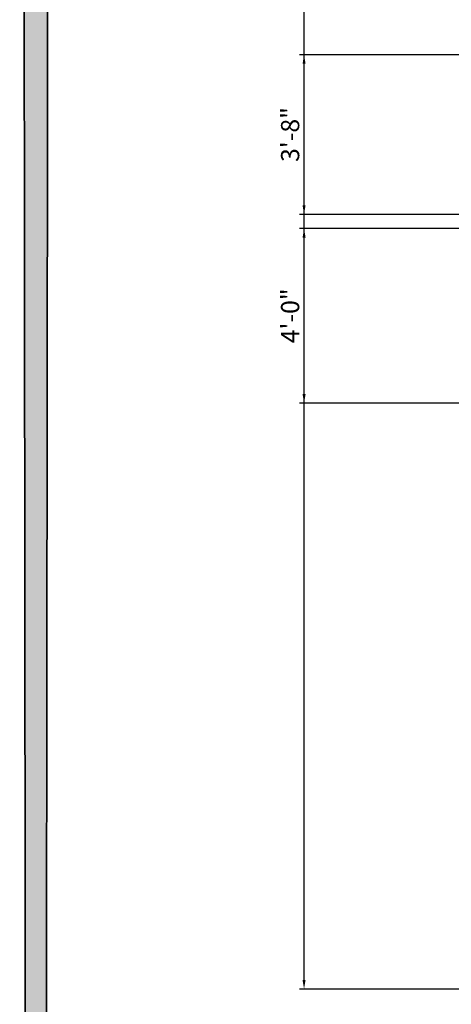
# Model space of a CAD drawing. Units: inches. Extents: x 1804 to 3296, y 909 to 2477.
# Tile 2 of 31: x 1804 to 1922, y 1059 to 1329. Entities that reach past the tile are written whole.
import ezdxf

# ---------------------------------------------------------------- set-up
doc = ezdxf.new("R2010")
doc.units = ezdxf.units.IN
doc.layers.add('A-ANNO-DIMS', color=2, linetype='Continuous', lineweight=18)
doc.layers.add('A-ANNO-TTLB', color=156, linetype='Continuous', lineweight=35)
doc.styles.get("Standard").update_dxf_attribs({"font": 'arial.ttf'})
doc.dimstyles.new('ISO-25', dxfattribs={"dimtxt": 5, "dimasz": 2.5, "dimexe": 1.25, "dimexo": 0.625, "dimtad": 1, "dimdec": 0, "dimlunit": 4, "dimtxsty": 'Standard', "dimcen": 2.5, "dimadec": 0, "dimazin": 0, "dimtfac": 1, "dimtdec": 0, "dimtmove": 0, "dimatfit": 3, "dimfxl": 1, "dimarcsym": 0})

# ---------------------------------------------------------------- blocks, each defined once
blk = doc.blocks.new('*D52')
at = {"layer": 'A-ANNO-DIMS', "color": 0, "lineweight": -2, "transparency": 16777216}
for p, q in [((1924.96, 1830.04), (1880.63, 1830.04)), ((1881.88, 1065.27), (1881.88, 1827.54)), ((1924.96, 1062.77), (1880.63, 1062.77))]:
    blk.add_line(p, q, dxfattribs=at)
at = {"layer": 'A-ANNO-DIMS', "color": 0, "lineweight": 100, "transparency": 16777216}
for points in [[(1881.47, 1827.54), (1882.3, 1827.54), (1881.88, 1830.04)], [(1881.47, 1065.27), (1882.3, 1065.27), (1881.88, 1062.77)]]:
    blk.add_solid(points, dxfattribs=at)
at = {"layer": 'Defpoints', "color": 0, "lineweight": 100, "transparency": 16777216}
for p in [(1881.88, 1830.04), (1925.58, 1830.04), (1925.58, 1062.77)]:
    blk.add_point(p, dxfattribs=at)
at = {"layer": 'A-ANNO-DIMS', "color": 0, "transparency": 16777216, "insert": (1878.67, 1446.4), "char_height": 5, "attachment_point": 5, "rotation": 90}
blk.add_mtext('63\'-11 1/2"', dxfattribs=at)
blk = doc.blocks.new('*D63')
at = {"layer": 'A-ANNO-DIMS', "color": 0, "lineweight": -2, "transparency": 16777216}
for p, q in [((2157.95, 1319.33), (1880.63, 1319.33)), ((1881.88, 1277.99), (1881.88, 1316.83)), ((2157.95, 1275.49), (1880.63, 1275.49))]:
    blk.add_line(p, q, dxfattribs=at)
at = {"layer": 'A-ANNO-DIMS', "color": 0, "lineweight": 100, "transparency": 16777216}
for points in [[(1881.47, 1316.83), (1882.3, 1316.83), (1881.88, 1319.33)], [(1881.47, 1277.99), (1882.3, 1277.99), (1881.88, 1275.49)]]:
    blk.add_solid(points, dxfattribs=at)
at = {"layer": 'Defpoints', "color": 0, "lineweight": 100, "transparency": 16777216}
for p in [(1881.88, 1319.33), (2158.58, 1319.33), (2158.58, 1275.49)]:
    blk.add_point(p, dxfattribs=at)
at = {"layer": 'A-ANNO-DIMS', "color": 0, "transparency": 16777216, "insert": (1878.7, 1297.41), "char_height": 5, "attachment_point": 5, "rotation": 90}
blk.add_mtext('3\'-8"', dxfattribs=at)
blk = doc.blocks.new('*D70')
at = {"layer": 'A-ANNO-DIMS', "color": 0, "lineweight": -2, "transparency": 16777216}
for p, q in [((2208.56, 1271.63), (1880.63, 1271.63)), ((1881.88, 1226.13), (1881.88, 1269.13)), ((2208.56, 1223.63), (1880.63, 1223.63))]:
    blk.add_line(p, q, dxfattribs=at)
at = {"layer": 'A-ANNO-DIMS', "color": 0, "lineweight": 100, "transparency": 16777216}
for points in [[(1881.47, 1269.13), (1882.3, 1269.13), (1881.88, 1271.63)], [(1881.47, 1226.13), (1882.3, 1226.13), (1881.88, 1223.63)]]:
    blk.add_solid(points, dxfattribs=at)
at = {"layer": 'Defpoints', "color": 0, "lineweight": 100, "transparency": 16777216}
for p in [(1881.88, 1271.63), (2209.19, 1271.63), (2209.19, 1223.63)]:
    blk.add_point(p, dxfattribs=at)
at = {"layer": 'A-ANNO-DIMS', "color": 0, "transparency": 16777216, "insert": (1878.7, 1247.63), "char_height": 5, "attachment_point": 5, "rotation": 90}
blk.add_mtext('4\'-0"', dxfattribs=at)

msp = doc.modelspace()

# ---------------------------------------------------------------- hatches: boundary and pattern name
at = {"layer": 'A-ANNO-TTLB'}
h = msp.add_hatch(color=256, dxfattribs=at)
h.dxf.hatch_style = 1
h.paths.add_polyline_path([(3294.53, 2476.54), (1803.79, 2476.54), (1805.43, 909.47), (3296.17, 909.47)])
h.paths.add_polyline_path([(1811, 914.33), (1812.79, 2467.54), (3285.53, 2467.54), (3283.74, 914.33)], flags=16)
h.paths.add_polyline_path([(1925.58, 1062.77), (1925.58, 1138.07), (1925.58, 1539.88), (1925.58, 1793.38), (1925.58, 1830.04), (2325.54, 1830.04), (2325.54, 1793.38), (2325.54, 1586.42), (2325.54, 1138.07), (2325.54, 1062.77)], flags=0)
h.paths.add_polyline_path([(1997.22, 1029.4), (2008.85, 1037.96), (2008.85, 1020.84)], flags=0)
h.paths.add_polyline_path([(1934.58, 1138.07), (1934.58, 1147.07), (2078.77, 1147.07), (2078.77, 1138.07), (2060.94, 1138.07)], flags=0)
h.paths.add_polyline_path([(1944.35, 1138.07), (1944.35, 1147.07), (2056.05, 1147.07), (2056.05, 1138.07)], flags=0)
h.paths.add_polyline_path([(2222.24, 1037.96), (2233.87, 1029.4), (2222.24, 1020.84)], flags=0)
h.paths.add_polyline_path([(2061.94, 1139.07), (2061.94, 1146.07), (2077.77, 1146.07), (2077.77, 1139.07)], flags=0)
h.paths.add_polyline_path([(2149.58, 1138.07), (2149.58, 1269.44), (2158.58, 1269.44), (2158.58, 1326.69), (2149.58, 1326.69), (2149.58, 1340.94), (2139.6, 1340.94), (2139.6, 1434.25), (2149.58, 1434.25), (2149.58, 1447.36), (2158.58, 1447.36), (2158.58, 1423.87), (2158.58, 1408.06), (2198.46, 1408.06), (2198.46, 1412.56), (2282.65, 1412.56), (2282.65, 1465.94), (2316.54, 1465.94), (2316.54, 1590.92), (2192.86, 1590.92), (2192.86, 1595.3), (2291.17, 1595.3), (2291.17, 1590.92), (2316.54, 1590.92), (2316.54, 1784.38), (2300.24, 1784.38), (2300.24, 1757.47), (2268, 1757.47), (2268, 1681.04), (2180.87, 1681.04), (2180.87, 1757.47), (2148.63, 1757.47), (2148.63, 1784.38), (2119.08, 1784.38), (2119.08, 1585.58), (2114.58, 1585.58), (2114.58, 1784.38), (2064.11, 1784.38), (2046.28, 1784.38), (2046.28, 1760.38), (1958.58, 1760.38), (1958.58, 1664.38), (1934.58, 1664.38), (1934.58, 1784.38), (1934.58, 1793.38), (2046.28, 1793.38), (2064.11, 1793.38), (2119.08, 1793.38), (2230.78, 1793.38), (2230.78, 1784.38), (2268, 1784.38), (2300.24, 1784.38), (2316.54, 1784.38), (2316.54, 1590.92), (2316.54, 1373.73), (2316.54, 1138.07)], flags=0)
h.paths.add_polyline_path([(2209.19, 1166.63), (2209.19, 1175.63), (2158.58, 1175.63), (2209.19, 1223.63), (2209.19, 1231.63), (2183.88, 1231.63), (2183.88, 1301.66), (2242.59, 1301.66), (2242.59, 1326.69), (2316.54, 1326.69), (2272.59, 1271.63), (2272.59, 1223.63), (2316.54, 1175.63), (2272.59, 1175.63), (2272.59, 1166.63)], flags=0)
h.paths.add_polyline_path([(1947.77, 1345.22), (1947.77, 1457.48), (1991.2, 1457.48), (1991.2, 1451.7), (1991.2, 1352.18), (1991.2, 1345.22)], flags=0)
h.paths.add_polyline_path([(2209.19, 1271.63), (2262.59, 1271.63), (2262.59, 1311.85), (2272.59, 1301.66), (2272.59, 1271.63), (2269.92, 1269.63), (2270.59, 1269.63), (2270.59, 1225.63), (2211.19, 1225.63), (2211.19, 1269.63), (2211.86, 1269.63)], flags=0)
h.paths.add_polyline_path([(2000.34, 1378.21), (2000.34, 1429.71), (2025.22, 1429.71), (2025.22, 1378.21)], flags=0)
h.paths.add_polyline_path([(2001.34, 1379.21), (2001.34, 1428.71), (2024.22, 1428.71), (2024.22, 1379.21)], flags=0)
h.paths.add_polyline_path([(2012.34, 1390.21), (2012.34, 1417.71), (2013.22, 1417.71), (2013.22, 1390.21)], flags=0)
h.paths.add_polyline_path([(2237.56, 1331.19), (2237.56, 1340.18), (2238.62, 1340.18), (2238.62, 1386.84), (2241.04, 1386.84), (2242.06, 1386.84), (2242.06, 1408.06), (2316.54, 1331.19)], flags=0)
h.paths.add_polyline_path([(1953.73, 1464.35), (1953.73, 1498.59), (1981.74, 1498.59), (1981.74, 1464.35)], flags=0)
h.paths.add_polyline_path([(1987.63, 1462.08), (1987.63, 1500.95), (2104.07, 1500.95), (2104.07, 1462.08), (2099.27, 1462.08), (1993.6, 1462.08)], flags=0)
h.paths.add_polyline_path([(1956.06, 1481.47, -1), (1979.41, 1481.47, -1)], flags=0)
edge = h.paths.add_edge_path(flags=0)
edge.add_ellipse((2299.53, 1438.37), major_axis=(0.31, 21.36), ratio=0.670333, start_angle=0, end_angle=360)
h.paths.add_polyline_path([(2297.39, 1438.37, -1), (2301.67, 1438.37, -1)], flags=0)
h.paths.add_polyline_path([(2591.54, 1163.23), (2591.54, 1179.38), (2591.54, 1379.68), (2591.54, 1395.84), (2734.5, 1395.84), (2734.5, 1379.68), (2734.5, 1179.38), (2734.5, 1163.23)], flags=0)
h.paths.add_polyline_path([(2592.54, 1164.23), (2592.54, 1166.23), (2733.5, 1166.23), (2733.5, 1164.23)], flags=0)
h.paths.add_polyline_path([(2592.54, 1180.38), (2592.54, 1378.68), (2733.5, 1378.68), (2733.5, 1180.38)], flags=0)
h.paths.add_polyline_path([(2593.54, 1181.38), (2593.54, 1377.68), (2732.5, 1377.68), (2732.5, 1181.38)], flags=0)
h.paths.add_polyline_path([(2594.54, 1182.38), (2594.54, 1376.68), (2731.5, 1376.68), (2731.5, 1182.38)], flags=0)
h.paths.add_polyline_path([(1936.95, 1697.46), (1936.95, 1736.46), (1955.41, 1736.46), (1955.41, 1697.46)], flags=0)
h.paths.add_polyline_path([(1938.48, 1718.36), (1938.48, 1734.92), (1953.65, 1734.92), (1953.65, 1718.36)], flags=0)
h.paths.add_polyline_path([(1944.75, 1726.64, -1), (1947.37, 1726.64, -1)], flags=0)
h.paths.add_polyline_path([(2592.54, 1394.84), (2733.5, 1394.84), (2733.5, 1392.84), (2592.54, 1392.84)], flags=0)
h.paths.add_polyline_path([(1976.61, 1762.5), (1976.61, 1781.44), (2012.79, 1781.44), (2012.79, 1762.5)], flags=0)
h.paths.add_polyline_path([(1979.57, 1771.97, -1), (1991.39, 1771.97, -1)], flags=0)
h.paths.add_polyline_path([(1995.36, 1771.97, -1), (2007.18, 1771.97, -1)], flags=0)
h.paths.add_polyline_path([(2251.51, 1744.53), (2268, 1730.05), (2251.51, 1730.05)], flags=0)
h.paths.add_polyline_path([(2047.28, 1785.38), (2047.28, 1792.38), (2063.11, 1792.38), (2063.11, 1785.38)], flags=0)
h.paths.add_polyline_path([(2155.08, 1770.92, -1), (2174.42, 1770.92, -1)], flags=0)
h.paths.add_polyline_path([(2188.59, 1758.27), (2188.59, 1772.81), (2222.3, 1772.81), (2222.3, 1758.27)], flags=0)
h.paths.add_polyline_path([(2223.97, 1758.27), (2223.97, 1772.81), (2257.68, 1772.81), (2257.68, 1758.27)], flags=0)
h.paths.add_polyline_path([(2274.45, 1770.92, -1), (2293.8, 1770.92, -1)], flags=0)
h.paths.add_polyline_path([(2591.54, 1582.09), (2591.54, 1782.39), (2734.5, 1782.39), (2734.5, 1582.09)], flags=0)
h.paths.add_polyline_path([(2592.54, 1583.09), (2592.54, 1781.39), (2733.5, 1781.39), (2733.5, 1583.09)], flags=0)
h.paths.add_polyline_path([(2593.54, 1584.09), (2593.54, 1780.39), (2732.5, 1780.39), (2732.5, 1584.09)], flags=0)
h.paths.add_polyline_path([(2594.54, 1585.09), (2594.54, 1779.39), (2731.5, 1779.39), (2731.5, 1585.09)], flags=0)
h.paths.add_polyline_path([(1922.17, 1978.79), (1922.17, 2295.08), (1922.17, 2296.08), (2115.67, 2296.08), (2115.67, 2384.31), (2115.67, 2385.31), (2322.12, 2385.31), (2323.12, 2385.31), (2323.12, 1979.79), (2323.12, 1978.79), (1923.17, 1978.79)], flags=0)
h.paths.add_polyline_path([(1922.17, 1978.79), (1922.17, 2051.31), (1922.17, 2214.86), (1922.17, 2296.08), (2115.67, 2296.08), (2115.67, 2385.31), (2323.12, 2385.31), (2323.12, 2280.42), (2323.12, 1978.79), (2115.67, 1978.79)], flags=0)
h.paths.add_polyline_path([(1923.17, 1979.79), (1923.17, 2050.31), (2115.67, 2050.31), (2115.67, 2051.31), (1923.17, 2051.31), (1923.17, 2213.86), (1923.17, 2214.86), (1923.17, 2295.08), (1990.02, 2295.08), (1990.02, 2214.86), (1991.02, 2214.86), (1991.02, 2295.08), (2115.67, 2295.08), (2115.67, 1979.79), (2116.67, 1979.79), (2116.67, 2304.18), (2116.67, 2384.31), (2322.12, 2384.31), (2322.12, 2280.42), (2322.12, 1979.79), (2115.67, 1979.79)], flags=0)
h.paths.add_polyline_path([(2972.46, 1192.5), (2972.46, 1196.92), (2995.47, 1196.92), (2995.47, 1255.47), (2995.09, 1255.47), (2987.42, 1249.39), (2980.08, 1255.47), (2978.05, 1255.47), (2978.05, 1257.24), (2995.47, 1257.24), (2995.47, 1261.58), (3015.37, 1261.58), (3015.37, 1333.28), (3015.37, 1414.4), (3032.82, 1414.4), (3032.82, 1333.28), (3032.82, 1261.58), (3052.66, 1261.58), (3052.66, 1255.47), (3079.86, 1255.47), (3078.72, 1254.57), (3081.47, 1252.29), (3078.56, 1249.99), (3075.81, 1252.26), (3072.57, 1249.69), (3070.36, 1251.52), (3067.67, 1249.39), (3060.34, 1255.47), (3052.66, 1255.47), (3052.66, 1196.92), (3054.58, 1196.92), (3074, 1196.92), (3074, 1192.5), (3052.66, 1192.5), (2995.47, 1192.5)], flags=0)
h.paths.add_polyline_path([(2490.75, 1979.27), (2490.75, 1980.27), (2596.87, 1980.27), (2596.87, 2051.8), (2596.87, 2052.8), (2596.87, 2216.35), (2596.87, 2297.57), (2717.32, 2297.57), (2710.57, 2305.62), (2724.07, 2305.62), (2717.32, 2297.57), (2782.37, 2297.57), (2782.37, 2395.8), (3006.82, 2395.8), (3006.82, 1981.27), (3093.73, 1981.27), (3093.73, 1980.27), (3047.51, 1980.27), (3046.37, 1979.37), (3049.11, 1977.1), (3046.2, 1974.79), (3043.46, 1977.07), (3040.21, 1974.49), (3038, 1976.32), (3035.32, 1974.2), (3027.98, 1980.27), (2871.83, 1980.27), (2871.83, 1981.27), (2791.37, 1981.27), (2791.37, 2050.8), (2597.87, 2050.8), (2597.87, 1980.27), (2597.87, 1979.27), (2546.27, 1979.27), (2545.12, 1978.37), (2547.87, 1976.1), (2544.96, 1973.79), (2542.22, 1976.07), (2538.97, 1973.49), (2536.76, 1975.32), (2534.07, 1973.2), (2526.74, 1979.27)], flags=0)
h.paths.add_polyline_path([(2597.87, 2051.8), (2606.87, 2051.8), (2606.87, 2258.39), (2597.87, 2258.39), (2597.87, 2296.57), (2606.87, 2296.57), (2606.87, 2262.39), (2782.37, 2262.39), (2782.37, 2296.57), (2790.37, 2296.57), (2790.37, 2262.39), (2791.37, 2262.39), (2791.37, 2305.67), (2791.37, 2385.8), (2996.82, 2385.8), (2996.82, 2339.85), (3006.82, 2339.85), (3006.82, 2250.12), (2997.82, 2250.12), (2997.82, 1981.27), (2996.82, 1981.27), (2872.83, 1981.27), (2872.83, 1991.8), (2871.83, 1991.8), (2871.83, 2050.8), (2790.37, 2050.8), (2597.87, 2050.8)], flags=0)
h.paths.add_polyline_path([(2179.93, 2153.92), (2179.93, 2353.97), (2259.98, 2353.97), (2259.98, 2153.92)], flags=0)
h.paths.add_polyline_path([(2180.93, 2154.92), (2180.93, 2352.97), (2258.98, 2352.97), (2258.98, 2154.92)], flags=0)
h.paths.add_polyline_path([(2960.87, 1608.49), (2960.87, 1753.62), (3070.9, 1753.62), (3070.9, 1608.49)], flags=0)
h.paths.add_polyline_path([(2961.87, 1609.49), (2961.87, 1752.62), (3069.9, 1752.62), (3069.9, 1609.49)], flags=0)
h.paths.add_polyline_path([(2962.87, 1610.49), (2962.87, 1751.62), (3068.9, 1751.62), (3068.9, 1610.49)], flags=0)
h.paths.add_polyline_path([(2963.87, 1611.49), (2963.87, 1750.62), (3067.9, 1750.62), (3067.9, 1611.49)], flags=0)
h.paths.add_polyline_path([(2782.37, 2051.8), (2782.37, 2216.32), (2791.37, 2216.32), (2791.37, 2051.8), (2872.83, 2051.8), (2872.83, 2068.56), (2884.67, 2068.56), (2884.67, 2085.33), (2896.51, 2085.33), (2896.51, 2102.09), (2908.36, 2102.09), (2908.36, 2118.85), (2920.2, 2118.85), (2920.2, 2135.62), (2932.05, 2135.62), (2932.05, 2145.3), (2925.08, 2145.3), (2925.08, 2203.2), (2996.82, 2203.2), (2996.82, 2145.3), (2953.82, 2145.3), (2872.83, 2051.8), (2790.37, 2051.8)], flags=0)
h.paths.add_polyline_path([(2717.32, 2238.65), (2710.57, 2246.7), (2724.07, 2246.7)], flags=0)
h.paths.add_polyline_path([(2003.09, 1122.79), (2017.16, 1122.79), (2017.16, 1138.74), (2003.09, 1138.74)], flags=8)
h.paths.add_polyline_path([(2174.76, 1792.72), (2188.83, 1792.72), (2188.83, 1808.66), (2174.76, 1808.66)], flags=8)
h.paths.add_polyline_path([(1987.95, 1792.51), (2002.02, 1792.51), (2002.02, 1808.45), (1987.95, 1808.45)], flags=8)
h.paths.add_polyline_path([(2148.79, 1289.26), (2160.46, 1289.26), (2160.46, 1305.2), (2148.79, 1305.2)], flags=8)
h.paths.add_polyline_path([(2115.36, 1133.57), (2127.04, 1133.57), (2127.04, 1149.51), (2115.36, 1149.51)], flags=8)
h.paths.add_polyline_path([(2237.58, 1421.48), (2249.25, 1421.48), (2249.25, 1437.43), (2237.58, 1437.43)], flags=8)
h.paths.add_polyline_path([(2134.99, 1584.32), (2146.66, 1584.32), (2146.66, 1600.26), (2134.99, 1600.26)], flags=8)
h.paths.add_polyline_path([(2101.95, 1557.31), (2113.62, 1557.31), (2113.62, 1573.25), (2101.95, 1573.25)], flags=8)
h.paths.add_polyline_path([(2937.85, 1156.77), (3120.41, 1156.77), (3120.41, 1185.72), (2937.85, 1185.72)], flags=8)
h.paths.add_polyline_path([(2980.71, 1786.71), (3050.06, 1786.71), (3050.06, 1802.66), (2980.71, 1802.66)], flags=8)
h.paths.add_polyline_path([(2869.28, 1661.96), (2938.62, 1661.96), (2938.62, 1690.8), (2869.28, 1690.8)], flags=8)
h.paths.add_polyline_path([(3092.27, 1674.86), (3161.62, 1674.86), (3161.62, 1690.8), (3092.27, 1690.8)], flags=8)
h.paths.add_polyline_path([(2980.71, 1674.86), (3050.06, 1674.86), (3050.06, 1690.8), (2980.71, 1690.8)], flags=8)
h.paths.add_polyline_path([(2649.07, 1678.23), (2674.53, 1678.23), (2674.53, 1714.76), (2649.07, 1714.76)], flags=8)
h.paths.add_polyline_path([(2530.84, 1981.63), (2549.13, 1981.63), (2549.13, 1997.57), (2530.84, 1997.57)], flags=8)
h.paths.add_polyline_path([(3031.29, 1981.77), (3049.58, 1981.77), (3049.58, 1997.71), (3031.29, 1997.71)], flags=8)
h.paths.add_polyline_path([(2715.38, 1911.9), (2851.54, 1911.9), (2851.54, 1940.85), (2715.38, 1940.85)], flags=8)
h.paths.add_polyline_path([(2015.23, 1927.36), (2205.42, 1927.36), (2205.42, 1956.3), (2015.23, 1956.3)], flags=8)
h.paths.add_polyline_path([(2671.84, 2057.84), (2702.75, 2057.84), (2702.75, 2073.79), (2671.84, 2073.79)], flags=8)
h.paths.add_polyline_path([(2678.5, 2316.52), (2765.26, 2316.52), (2765.26, 2332.46), (2678.5, 2332.46)], flags=8)
h.paths.add_polyline_path([(2678.48, 2271.96), (2736.41, 2271.96), (2736.41, 2287.9), (2678.48, 2287.9)], flags=8)
h.paths.add_polyline_path([(2019.2, 972.79), (2243.21, 972.79), (2243.21, 1001.74), (2019.2, 1001.74)], flags=8)
h.paths.add_polyline_path([(2097.06, 1021.56), (2132.16, 1021.56), (2132.16, 1037.51), (2097.06, 1037.51)], flags=8)
h.paths.add_polyline_path([(2182.47, 1360.48), (2207.35, 1360.48), (2207.35, 1376.42), (2182.47, 1376.42)], flags=8)
h.paths.add_polyline_path([(2261.12, 1361.77), (2295.01, 1361.77), (2295.01, 1377.71), (2261.12, 1377.71)], flags=8)
h.paths.add_polyline_path([(2245.75, 1511.51), (2278.44, 1511.51), (2278.44, 1527.46), (2245.75, 1527.46)], flags=8)
h.paths.add_polyline_path([(1991.16, 1296.29), (2060.51, 1296.29), (2060.51, 1312.23), (1991.16, 1312.23)], flags=8)
h.paths.add_polyline_path([(2187, 1651.35), (2246.71, 1651.35), (2246.71, 1667.29), (2187, 1667.29)], flags=8)
h.paths.add_polyline_path([(1976.49, 1684.81), (2068.63, 1684.81), (2068.63, 1700.76), (1976.49, 1700.76)], flags=8)

# ---------------------------------------------------------------- linework, layer by layer
for points in [[(1803.79, 2476.54), (3294.53, 2476.54), (3296.17, 909.47), (1805.43, 909.47)], [(1812.79, 2467.54), (3285.53, 2467.54), (3283.74, 914.33), (1811, 914.33)]]:
    msp.add_lwpolyline(points, close=True, dxfattribs=at)

# ---------------------------------------------------------------- dimensions: what is measured, and where the dimension line sits
at = {"layer": 'A-ANNO-DIMS'}
for base, p1, p2, picture, middle in [((1881.88, 1830.04), (1925.58, 1062.77), (1925.58, 1830.04), '*D52', (1878.67, 1446.4)), ((1881.88, 1319.33), (2158.58, 1275.49), (2158.58, 1319.33), '*D63', (1878.7, 1297.41)), ((1881.88, 1271.63), (2209.19, 1223.63), (2209.19, 1271.63), '*D70', (1878.7, 1247.63))]:
    dim = msp.add_linear_dim(base=base, p1=p1, p2=p2, angle=90, dimstyle='ISO-25', override={"dimdec": 1, "dimlfac": 1, "dimrnd": 0, "dimzin": 1, "dimdsep": 46, "dimlunit": 4, "dimfrac": 2}, dxfattribs=at)
    dim.commit()
    dim.dimension.update_dxf_attribs({"geometry": picture, "text_midpoint": middle})

doc.saveas('drawing.dxf')
